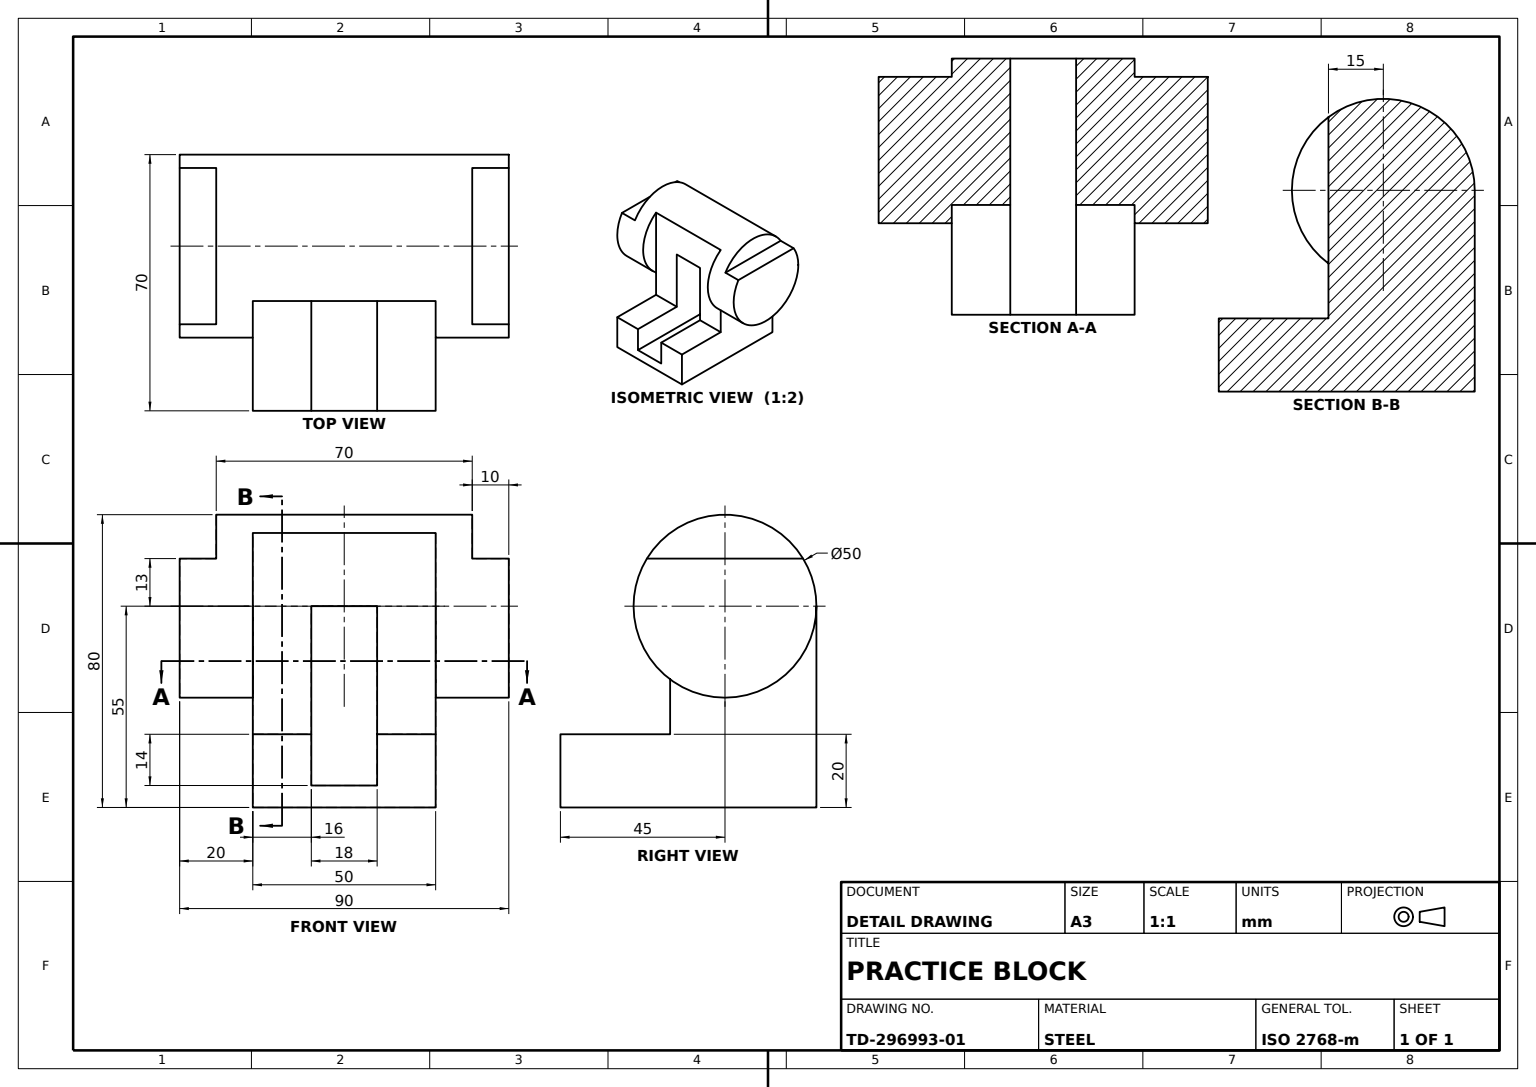
SolidWorks part; units mm, degrees
material "Plain Carbon Steel"
ref_plane "Front Plane" through (0, 0, 0) normal (0, 0, 1) x (1, 0, 0)
ref_plane "Top Plane" through (0, 0, 0) normal (0, 1, 0) x (1, 0, 0)
ref_plane "Right Plane" through (0, 0, 0) normal (1, 0, 0) x (0, 0, -1)
sketch "U Base Profile Sketch" plane through (0, 0, 0) normal (1, 0, 0) x (0, 0, -1)
  line L0 (25, 0) -> (-25, 0)
  line L1 (-25, 0) -> (-25, 20)
  line L2 (-25, 20) -> (-9, 20)
  line L3 (-9, 20) -> (-9, 6)
  line L4 (-9, 6) -> (9, 6)
  line L5 (9, 6) -> (9, 20)
  line L6 (9, 20) -> (25, 20)
  line L7 (25, 20) -> (25, 0)
  point P4 (0, 0)
  dimension "D1" = 25
  dimension "D2" = 20
  dimension "D3" = 14
  dimension "D4" = 16
  dimension "D5" = 18
  dimension "D6" = 20
extrude "U Base" add sketch "U Base Profile Sketch" along normal blind 20
sketch "Upright Web Sketch" plane through (0, 0, 0) normal (-1, 0, 0) x (0, 0, 1)
  line L1 (25, 20) -> (-25, 20)
  line L2 (25, 20) -> (25, 70)
  line L3 (25, 70) -> (-25, 70)
  line L4 (-25, 20) -> (-25, 70)
  line L5 (9, 20) -> (-9, 20)
  line L6 (9, 20) -> (9, 65)
  line L7 (9, 65) -> (-9, 65)
  line L8 (-9, 20) -> (-9, 65)
  line L9 (-25, 20) -> (25, 20)
  line L10 (-25, 20) -> (-25, 0)
  line L11 (-25, 0) -> (25, 0)
  line L12 (25, 20) -> (25, 0)
  line M4 (9, 20) -> (9, 6)
  line M5 (9, 6) -> (-9, 6)
  line M6 (-9, 6) -> (-9, 20)
  line M7 (-9, 20) -> (-25, 20)
  line M8 (-25, 20) -> (-25, 0)
  line M9 (-25, 0) -> (25, 0)
  line M10 (25, 0) -> (25, 20)
  line M11 (25, 20) -> (9, 20)
  dimension "D1" = 50
  dimension "D2" = 18
  dimension "D3" = 45
extrude "Upright Web" add sketch "Upright Web Sketch" along normal blind 50 contours L8 L7 L6 L2 L3 L4 M7 M11 | M11 M4 M5 M6 M7 M8 M9 M10
sketch "Cylinder Ø50 Sketch" plane through (0, 0, 25) normal (0, 0, 1) x (1, 0, 0)
  line L0 (-50, 0) -> (-50, 70) construction
  circle A0 centre (-25, 55) radius 25
  dimension "D1" = 50
  dimension "D2" = 25
  dimension "D3" = 55
extrude "Cylinder Ø50" add sketch "Cylinder Ø50 Sketch" against normal blind 50
sketch "Web Clearance Cut Sketch" plane through (0, 0, 25) normal (0, 0, 1) x (1, 0, 0)
  line L0 (-50, 55) -> (-50, 70)
  line L1 (-50, 70) -> (-45, 70)
  line L2 (-5, 70) -> (0, 70)
  line L3 (0, 70) -> (0, 55)
  circle A0 centre (-25, 55) radius 25
  line M3 (0, 20) -> (0, 70)
  line M4 (0, 70) -> (-5, 70)
  line M6 (-45, 70) -> (-50, 70)
  line M7 (-50, 70) -> (-50, 0)
  dimension "D1" = 50
  dimension "D2" = 15
  dimension "D3" = 25
extrude "Web Clearance Cut" cut sketch "Web Clearance Cut Sketch" against normal blind 50 contours A0 M6 M7 | A0 M3 M4
sketch "Side Relief Cut Sketch" plane through (0, 0, 0) normal (1, 0, 0) x (0, 0, -1)
  line L1 (-9, 55) -> (9, 55)
  line L2 (-9, 55) -> (-9, 20)
  line L3 (-9, 20) -> (9, 20)
  line L4 (9, 55) -> (9, 20)
extrude "Side Relief Cut" cut sketch "Side Relief Cut Sketch" against normal blind 50
sketch "Base Slot Cut Sketch" plane through (0, 0, 0) normal (1, 0, 0) x (0, 0, -1)
  line L0 (25, 55) -> (25, 80) construction
  line L1 (-25, 20) -> (25, 20)
  line L2 (-25, 20) -> (-25, 70)
  line L3 (-25, 70) -> (25, 70)
  line L4 (25, 20) -> (25, 70)
extrude "Base Slot Cut" cut sketch "Base Slot Cut Sketch" against normal blind 10
sketch "Web Slot Cut Sketch" plane through (0, 70, 0) normal (0, -1, 0) x (1, 0, 0)
  line L1 (-5, 25) -> (-10, 25)
  line L2 (-5, 25) -> (-5, -25)
  line L3 (-5, -25) -> (-10, -25)
  line L4 (-10, 25) -> (-10, -25)
extrude "Web Slot Cut" cut sketch "Web Slot Cut Sketch" against normal blind 10
sketch "End Boss A Sketch" plane through (0, 0, 25) normal (0, 0, 1) x (1, 0, 0)
  circle A0 centre (-25, 55) radius 25
  dimension "D1" = 50
extrude "End Boss A Ø50" add sketch "End Boss A Sketch" along normal blind 20
sketch "End Boss B Sketch" plane through (0, 0, -25) normal (0, 0, -1) x (-1, 0, 0)
  circle A0 centre (25, 55) radius 25
  dimension "D1" = 50
extrude "End Boss B Ø50" add sketch "End Boss B Sketch" along normal blind 20
sketch "End Slot A Sketch" plane through (0, 0, 45) normal (0, 0, 1) x (1, 0, 0)
  line L0 (-46.3542, 68) -> (-3.6458, 68)
  circle A0 centre (-25, 55) radius 25 construction
  arc A1 (-3.6458, 68) -> (-46.3542, 68) centre (-25, 55) ccw
  dimension "D2" = 50
  dimension "D1" = 13
extrude "End Slot A" cut sketch "End Slot A Sketch" against normal blind 10
sketch "End Slot B Sketch" plane through (0, 0, -45) normal (0, 0, -1) x (-1, 0, 0)
  line L0 (3.6458, 68) -> (46.3542, 68)
  circle A0 centre (25, 55) radius 25 construction
  arc A1 (46.3542, 68) -> (3.6458, 68) centre (25, 55) ccw
  dimension "D2" = 50
  dimension "D1" = 13
extrude "End Slot B" cut sketch "End Slot B Sketch" against normal blind 10
